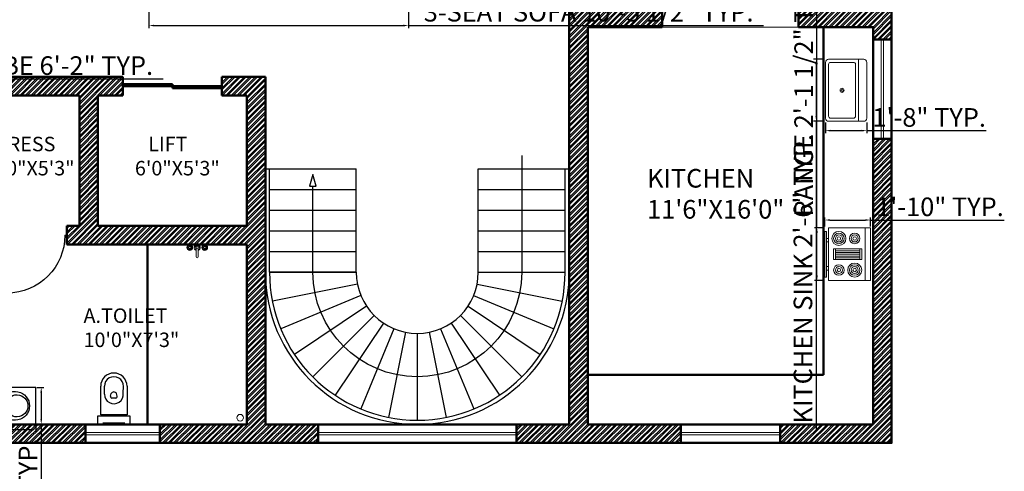
# Model space of a CAD drawing. Units: inches. Extents: x 3590 to 5167, y 65 to 1917.
# Tile 19 of 100: x 3884 to 4360, y 1312 to 1531. Entities that reach past the tile are written whole.
import ezdxf

# ---------------------------------------------------------------- set-up
doc = ezdxf.new("R2010")
doc.units = ezdxf.units.IN
doc.linetypes.add('DASHED', pattern=[0.75, 0.5, -0.25])
for name, color, linetype, lineweight in [('A-ANNO-DIMS', 2, 'Continuous', 18), ('A-AREA-IDEN', 7, 'Continuous', 18), ('A-DOOR', 3, 'Continuous', 25), ('A-FLOR-FIXT', 8, 'Continuous', 18), ('A-FLOR-STRS', 7, 'Continuous', 25), ('A-GLAZ', 4, 'Continuous', 18), ('A-WALL', 7, 'Continuous', 50), ('A-WALL-PATT', 251, 'Continuous', 13), ('S-BEAM-OVHD', 7, 'DASHED', 18)]:
    doc.layers.add(name, color=color, linetype=linetype, lineweight=lineweight)
doc.layers.add('SANTEH', color=7, linetype='Continuous')
doc.styles.get("Standard").update_dxf_attribs({"font": 'arial.ttf'})
doc.dimstyles.new('ISO-25', dxfattribs={"dimtxt": 9, "dimasz": 2.5, "dimexe": 1.25, "dimexo": 0.625, "dimtad": 1, "dimdec": 1, "dimlunit": 3, "dimtxsty": 'Standard', "dimcen": 2.5, "dimadec": 0, "dimazin": 0, "dimtfac": 1, "dimtdec": 1, "dimtmove": 0, "dimatfit": 3, "dimfxl": 1, "dimarcsym": 0})

# ---------------------------------------------------------------- blocks, each defined once
blk = doc.blocks.new('*U1')
blk.add_line((-21, 0), (21, 0))
blk = doc.blocks.new('*U2')
at = {"layer": 'A-FLOR-STRS', "color": 0, "linetype": 'ByBlock', "lineweight": -2, "transparency": 16777216}
for p, rotation in [((4066.16, 1458.03), 101.2499999999998), ((4076.01, 1459), 89.99999999999982), ((4085.86, 1458.03), 78.7499999999998), ((4056.69, 1455.15), 112.4999999999998), ((4095.34, 1455.15), 67.4999999999998), ((4047.96, 1450.49), 123.7499999999997), ((4104.07, 1450.49), 56.24999999999984), ((4040.3, 1444.21), 134.9999999999996), ((4111.72, 1444.21), 44.99999999999992), ((4034.02, 1436.56), 146.2499999999996), ((4118, 1436.56), 33.74999999999991), ((4029.36, 1427.82), 157.4999999999995), ((4122.67, 1427.82), 22.49999999999996), ((4026.48, 1418.35), 168.7499999999995), ((4125.54, 1418.35), 11.25), ((4025.51, 1408.5), 180)]:
    blk.add_blockref('*U1', p, dxfattribs=dict(at, rotation=rotation))
blk.add_blockref('*U1', (4126.51, 1408.5), dxfattribs=at)
blk = doc.blocks.new('Range-Oven - 30 in top')
for p, q in [((0, -3), (30, -3)), ((12, -6), (18, -6)), ((13, -20), (13, -6)), ((14, -6), (14, -20)), ((15, -20), (15, -6)), ((16, -6), (16, -20)), ((17, -20), (17, -6)), ((18, -20), (12, -20)), ((6, -24), (6, -25)), ((8, -25), (8, -24)), ((22, -25), (22, -24)), ((24, -24), (24, -25))]:
    blk.add_line(p, q)
for points in [[(0, -24), (0, 0), (30, 0), (30, -24)], [(12, -21), (12, -5), (18, -5), (18, -21)], [(2, -26), (2, -25), (28, -25), (28, -26)]]:
    blk.add_lwpolyline(points, close=True)
for centre, radius in [((6, -9), 4), ((6, -9), 3), ((6, -9), 2), ((6, -9), 1), ((24, -9), 3), ((24, -9), 2), ((24, -9), 1), ((6, -18), 3), ((6, -18), 2), ((24, -18), 4), ((24, -18), 3), ((24, -18), 2), ((6, -18), 1), ((24, -18), 1)]:
    blk.add_circle(centre, radius)
blk = doc.blocks.new('Sink-single - 30 in top')
blk.add_line((-15, -3.999996), (15, -3.999996))
for points in [[(-13.5, 0), (13.5, 0)], [(-15, -18.499996), (-15, -1.5)], [(15, -1.5), (15, -18.499996)], [(-13.5, -17.499996), (-13.5, -6.499996)], [(-12.5, -5.499996), (12.5, -5.499996)], [(13.5, -6.499996), (13.5, -17.499996)], [(12.5, -18.499996), (-12.5, -18.499996)], [(13.5, -19.999996), (-13.5, -19.999996)]]:
    blk.add_lwpolyline(points)
for radius in [1, 0.5]:
    blk.add_circle((0, -11.999996), radius)
for centre, radius, start, end in [((-13.5, -1.5), 1.5, 90, 180), ((13.5, -1.5), 1.5, 0, 90), ((-12.5, -6.499996), 1, 90, 180), ((12.5, -6.499996), 1, 0, 90), ((-13.5, -18.499996), 1.5, 180, 270), ((-12.5, -17.499996), 1, 180, 270), ((12.5, -17.499996), 1, 270, 0), ((13.5, -18.499996), 1.5, 270, 0)]:
    blk.add_arc(centre, radius, start, end)
blk = doc.blocks.new('D2')
for p, q in [((1, 0), (1, 28)), ((2, 0), (2, 27.98)), ((0, 0), (2, 0)), ((29, 0), (30, 0))]:
    blk.add_line(p, q)
at = {"ltscale": 0.5}
blk.add_arc((1, 0), 28, 0, 90, dxfattribs=at)
blk = doc.blocks.new('y3')
at = {"layer": 'SANTEH', "ltscale": 5}
for p, q in [((38, 131), (38, 521)), ((88, 411), (88, 521)), ((172, 385), (181, 421)), ((263, 385), (254, 421)), ((347, 426), (348, 521)), ((398, 521), (398, 131)), ((244, 358), (191, 358)), ((398, 131), (38, 131)), ((67, 21), (367, 21))]:
    blk.add_line(p, q, dxfattribs=at)
blk.add_lwpolyline([(0, 115), (435, 115), (435, 0), (0, 0), (0, 115)], dxfattribs=at)
for centre, radius, start, end in [((218, 521), 180, 0, 180), ((218, 521), 130, 359.1579, 180), ((218, 411), 130, 180, 5.9855), ((218, 400), 42.2, 30.5234, 149.4766), ((191, 378), 20, 160.5038, 270), ((244, 378), 20, 270, 19.4962)]:
    blk.add_arc(centre, radius, start, end, dxfattribs=at)
blk = doc.blocks.new('r11')
at = {"layer": 'SANTEH', "ltscale": 5}
for p, q in [((0, 0), (600, 0)), ((0, -600), (0, 0)), ((600, 0), (600, -600)), ((210, -50), (390, -50)), ((210, -50), (210, -50)), ((224, -63), (376, -63)), ((224, -113), (224, -63)), ((376, -113), (224, -113)), ((233, -79), (249, -69)), ((233, -98), (233, -79)), ((249, -107), (233, -98)), ((249, -69), (266, -79)), ((266, -98), (249, -107)), ((266, -79), (266, -98)), ((288, -202), (288, -113)), ((312, -113), (312, -202)), ((334, -79), (351, -69)), ((334, -98), (334, -79)), ((351, -107), (334, -98)), ((351, -69), (367, -79)), ((367, -98), (351, -107)), ((367, -79), (367, -98)), ((376, -63), (376, -113)), ((312, -184), (288, -184)), ((312, -202), (288, -202)), ((600, -600), (0, -600))]:
    blk.add_line(p, q, dxfattribs=at)
for centre, radius, start, end in [((300, -266), 234, 112.5, 67.5), ((300, -293), 180, 93.8183, 86.1817)]:
    blk.add_arc(centre, radius, start, end, dxfattribs=at)
blk = doc.blocks.new('Faucet - Bathroom top')
for p, q in [((-4.107, 0.125), (-4.375, 0.125)), ((-3.75, 0.4788), (-3.75, 0.75)), ((-3.5, 0.482), (-3.5, 0.75)), ((-3.1461, 0.125), (-2.875, 0.125)), ((3.143, 0.125), (2.875, 0.125)), ((3.5, 0.4788), (3.5, 0.75)), ((3.75, 0.482), (3.75, 0.75)), ((4.1039, 0.125), (4.375, 0.125)), ((-4.1039, -0.125), (-4.375, -0.125)), ((-3.75, -0.4821), (-3.75, -0.75)), ((-3.5, -0.4789), (-3.5, -0.75)), ((-3.143, -0.125), (-2.875, -0.125)), ((-0.5, -0.8639), (-0.5, -4.5)), ((0.5, -4.5), (0.5, -0.8631)), ((3.1461, -0.125), (2.875, -0.125)), ((3.5, -0.4821), (3.5, -0.75)), ((3.75, -0.4789), (3.75, -0.75)), ((4.107, -0.125), (4.375, -0.125))]:
    blk.add_line(p, q)
for centre, radius in [((-3.625, 0), 1.375), ((-4.625, 0), 0.2795), ((-3.625, 0), 0.5), ((-3.625, 1), 0.2795), ((-2.625, 0), 0.2795), ((0, 0), 0.5), ((3.625, 0), 1.375), ((2.625, 0), 0.2795), ((3.625, 0), 0.5), ((3.625, 1), 0.2795), ((4.625, 0), 0.2795), ((-3.625, -1), 0.2795), ((3.625, -1), 0.2795)]:
    blk.add_circle(centre, radius)
for centre, radius, start, end in [((-3.625, 0), 1, 105.2407, 164.2093), ((-3.625, 0), 1, 16.44125, 74.07887), ((0, 0), 1.5, 289.6514, 250.3603), ((0, 0), 1, 300.3431, 239.7554), ((3.625, 0), 1, 106.12, 164.0884), ((3.625, 0), 1, 16.23422, 73.90469), ((-3.625, 0), 1, 196.2342, 253.9047), ((-3.625, 0), 1, 286.12, 344.0884), ((0, -4.5), 0.5, 180, 0), ((3.625, 0), 1, 196.4413, 254.0789), ((3.625, 0), 1, 285.2407, 344.2093)]:
    blk.add_arc(centre, radius, start, end)
blk = doc.blocks.new('*D290')
at = {"layer": 'A-ANNO-DIMS', "color": 0, "lineweight": -2, "transparency": 16777216}
for p, q in [((3742.44, 1491.53), (3742.44, 1503.26)), ((3744.94, 1502.01), (3813.99, 1502.01)), ((3816.49, 1491.53), (3816.49, 1503.26)), ((3816.49, 1502.01), (3953, 1502.01))]:
    blk.add_line(p, q, dxfattribs=at)
at = {"layer": 'A-ANNO-DIMS', "color": 0, "transparency": 16777216}
for points in [[(3744.94, 1502.43), (3744.94, 1501.59), (3742.44, 1502.01)], [(3813.99, 1502.43), (3813.99, 1501.59), (3816.49, 1502.01)]]:
    blk.add_solid(points, dxfattribs=at)
at = {"layer": 'Defpoints', "color": 0, "transparency": 16777216}
for p in [(3816.49, 1502.01), (3742.44, 1490.9), (3816.49, 1490.9)]:
    blk.add_point(p, dxfattribs=at)
at = {"layer": 'A-ANNO-DIMS', "color": 0, "transparency": 16777216, "insert": (3885.99, 1507.29), "char_height": 9, "attachment_point": 5}
blk.add_mtext('WARDROBE 6\'-2" TYP.', dxfattribs=at)
blk = doc.blocks.new('*D294')
at = {"layer": 'A-ANNO-DIMS', "color": 0, "lineweight": -2, "transparency": 16777216}
for p, q in [((3946.19, 1546.03), (3946.19, 1526.56)), ((4071.76, 1546.03), (4071.76, 1526.56)), ((3948.69, 1527.81), (4069.26, 1527.81)), ((4071.76, 1527.81), (4243.57, 1527.81))]:
    blk.add_line(p, q, dxfattribs=at)
at = {"layer": 'A-ANNO-DIMS', "color": 0, "transparency": 16777216}
for points in [[(3948.69, 1528.23), (3948.69, 1527.4), (3946.19, 1527.81)], [(4069.26, 1528.23), (4069.26, 1527.4), (4071.76, 1527.81)]]:
    blk.add_solid(points, dxfattribs=at)
at = {"layer": 'Defpoints', "color": 0, "transparency": 16777216}
for p in [(3946.19, 1546.65), (4071.76, 1546.65), (4071.76, 1527.81)]:
    blk.add_point(p, dxfattribs=at)
at = {"layer": 'A-ANNO-DIMS', "color": 0, "transparency": 16777216, "insert": (4158.91, 1533.1), "char_height": 9, "attachment_point": 5}
blk.add_mtext('3-SEAT SOFA 10\'-5 1/2" TYP.', dxfattribs=at)
blk = doc.blocks.new('*D306')
at = {"layer": 'A-ANNO-DIMS', "color": 0, "lineweight": -2, "transparency": 16777216}
for p, q in [((3892, 1352.87), (3895.31, 1352.87)), ((3894.06, 1350.37), (3894.06, 1337.5)), ((3892, 1335), (3895.31, 1335)), ((3894.06, 1335), (3894.06, 1193.58))]:
    blk.add_line(p, q, dxfattribs=at)
at = {"layer": 'A-ANNO-DIMS', "color": 0, "transparency": 16777216}
for points in [[(3893.64, 1350.37), (3894.48, 1350.37), (3894.06, 1352.87)], [(3893.64, 1337.5), (3894.48, 1337.5), (3894.06, 1335)]]:
    blk.add_solid(points, dxfattribs=at)
at = {"layer": 'Defpoints', "color": 0, "transparency": 16777216}
for p in [(3891.38, 1352.87), (3891.38, 1335), (3894.06, 1335)]:
    blk.add_point(p, dxfattribs=at)
at = {"layer": 'A-ANNO-DIMS', "color": 0, "transparency": 16777216, "insert": (3888.78, 1263.04), "char_height": 9, "attachment_point": 5, "rotation": 90}
blk.add_mtext('WASH BASIN 1\'-6" TYP.', dxfattribs=at)
blk = doc.blocks.new('*D307')
at = {"layer": 'A-ANNO-DIMS', "color": 0, "lineweight": -2, "transparency": 16777216}
for p, q in [((3873.51, 1334.37), (3873.51, 1331.07)), ((3891.38, 1334.37), (3891.38, 1331.07)), ((3873.51, 1332.32), (3815.75, 1332.32)), ((3888.88, 1332.32), (3876.01, 1332.32))]:
    blk.add_line(p, q, dxfattribs=at)
at = {"layer": 'A-ANNO-DIMS', "color": 0, "transparency": 16777216}
for points in [[(3876.01, 1332.74), (3876.01, 1331.9), (3873.51, 1332.32)], [(3888.88, 1332.74), (3888.88, 1331.9), (3891.38, 1332.32)]]:
    blk.add_solid(points, dxfattribs=at)
at = {"layer": 'Defpoints', "color": 0, "transparency": 16777216}
for p in [(3873.51, 1335), (3891.38, 1335), (3873.51, 1332.32)]:
    blk.add_point(p, dxfattribs=at)
at = {"layer": 'A-ANNO-DIMS', "color": 0, "transparency": 16777216, "insert": (3843.38, 1337.54), "char_height": 9, "attachment_point": 5}
blk.add_mtext('1\'-6" TYP.', dxfattribs=at)
blk = doc.blocks.new('*D308')
at = {"layer": 'A-ANNO-DIMS', "color": 0, "lineweight": -2, "transparency": 16777216}
for p, q in [((4269.39, 1429.97), (4269.39, 1557.29)), ((4272.58, 1429.97), (4268.14, 1429.97)), ((4269.39, 1407.01), (4269.39, 1427.47)), ((4272.58, 1404.51), (4268.14, 1404.51))]:
    blk.add_line(p, q, dxfattribs=at)
at = {"layer": 'A-ANNO-DIMS', "color": 0, "transparency": 16777216}
for points in [[(4268.97, 1427.47), (4269.8, 1427.47), (4269.39, 1429.97)], [(4268.97, 1407.01), (4269.8, 1407.01), (4269.39, 1404.51)]]:
    blk.add_solid(points, dxfattribs=at)
at = {"layer": 'Defpoints', "color": 0, "transparency": 16777216}
for p in [(4269.39, 1429.97), (4273.2, 1429.97), (4273.2, 1404.51)]:
    blk.add_point(p, dxfattribs=at)
at = {"layer": 'A-ANNO-DIMS', "color": 0, "transparency": 16777216, "insert": (4264.11, 1494.88), "char_height": 9, "attachment_point": 5, "rotation": 90}
blk.add_mtext('RANGE 2\'-1 1/2" TYP.', dxfattribs=at)
blk = doc.blocks.new('*D309')
at = {"layer": 'A-ANNO-DIMS', "color": 0, "lineweight": -2, "transparency": 16777216}
for p, q in [((4273.2, 1430.59), (4273.2, 1435.04)), ((4295.27, 1430.59), (4295.27, 1435.04)), ((4275.7, 1433.79), (4292.77, 1433.79)), ((4295.27, 1433.79), (4360.02, 1433.79))]:
    blk.add_line(p, q, dxfattribs=at)
at = {"layer": 'A-ANNO-DIMS', "color": 0, "transparency": 16777216}
for points in [[(4275.7, 1434.2), (4275.7, 1433.37), (4273.2, 1433.79)], [(4292.77, 1434.2), (4292.77, 1433.37), (4295.27, 1433.79)]]:
    blk.add_solid(points, dxfattribs=at)
at = {"layer": 'Defpoints', "color": 0, "transparency": 16777216}
for p in [(4273.2, 1429.97), (4295.27, 1433.79), (4295.27, 1429.97)]:
    blk.add_point(p, dxfattribs=at)
at = {"layer": 'A-ANNO-DIMS', "color": 0, "transparency": 16777216, "insert": (4328.89, 1439.01), "char_height": 9, "attachment_point": 5}
blk.add_mtext('1\'-10" TYP.', dxfattribs=at)
blk = doc.blocks.new('*D310')
at = {"layer": 'A-ANNO-DIMS', "color": 0, "lineweight": -2, "transparency": 16777216}
for p, q in [((4272.91, 1511.51), (4267.78, 1511.51)), ((4269.03, 1509.01), (4269.03, 1484.01)), ((4272.91, 1481.51), (4267.78, 1481.51)), ((4269.03, 1481.51), (4269.03, 1331.79))]:
    blk.add_line(p, q, dxfattribs=at)
at = {"layer": 'A-ANNO-DIMS', "color": 0, "transparency": 16777216}
for points in [[(4268.62, 1509.01), (4269.45, 1509.01), (4269.03, 1511.51)], [(4268.62, 1484.01), (4269.45, 1484.01), (4269.03, 1481.51)]]:
    blk.add_solid(points, dxfattribs=at)
at = {"layer": 'Defpoints', "color": 0, "transparency": 16777216}
for p in [(4273.53, 1511.51), (4269.03, 1481.51), (4273.53, 1481.51)]:
    blk.add_point(p, dxfattribs=at)
at = {"layer": 'A-ANNO-DIMS', "color": 0, "transparency": 16777216, "insert": (4263.76, 1405.4), "char_height": 9, "attachment_point": 5, "rotation": 90}
blk.add_mtext('KITCHEN SINK 2\'-6" TYP.', dxfattribs=at)
blk = doc.blocks.new('*D311')
at = {"layer": 'A-ANNO-DIMS', "color": 0, "lineweight": -2, "transparency": 16777216}
for p, q in [((4273.53, 1480.89), (4273.53, 1475.76)), ((4276.03, 1477.01), (4291.03, 1477.01)), ((4293.53, 1480.89), (4293.53, 1475.76)), ((4293.53, 1477.01), (4351.3, 1477.01))]:
    blk.add_line(p, q, dxfattribs=at)
at = {"layer": 'A-ANNO-DIMS', "color": 0, "transparency": 16777216}
for points in [[(4276.03, 1477.43), (4276.03, 1476.6), (4273.53, 1477.01)], [(4291.03, 1477.43), (4291.03, 1476.6), (4293.53, 1477.01)]]:
    blk.add_solid(points, dxfattribs=at)
at = {"layer": 'Defpoints', "color": 0, "transparency": 16777216}
for p in [(4273.53, 1481.51), (4293.53, 1481.51), (4293.53, 1477.01)]:
    blk.add_point(p, dxfattribs=at)
at = {"layer": 'A-ANNO-DIMS', "color": 0, "transparency": 16777216, "insert": (4323.67, 1482.23), "char_height": 9, "attachment_point": 5}
blk.add_mtext('1\'-8" TYP.', dxfattribs=at)

msp = doc.modelspace()

# ---------------------------------------------------------------- hatches: boundary and pattern name
at = {"layer": 'A-WALL-PATT', "transparency": 33554687}
h = msp.add_hatch(dxfattribs=at)
h.set_pattern_fill('ANSI32', color=256, scale=0.2)
h.paths.add_polyline_path([(3768.51, 1806), (3645.51, 1806), (3645.51, 1785), (3654.51, 1785), (3654.51, 1797), (3671.16, 1797), (3768.51, 1797)])
h.paths.add_polyline_path([(3909.51, 1806), (3816.51, 1806), (3816.51, 1797), (3864.51, 1797), (3864.51, 1791), (3873.51, 1791), (3873.51, 1797), (3909.51, 1797)])
h.paths.add_polyline_path([(4053.51, 1806), (3969.51, 1806), (3969.51, 1797), (4053.51, 1797)])
h.paths.add_polyline_path([(4215.51, 1806), (4113.51, 1806), (4113.51, 1797), (4206.51, 1797), (4206.51, 1791), (4215.51, 1791)])
h.paths.add_polyline_path([(3654.51, 1737), (3645.51, 1737), (3645.51, 1620), (3654.51, 1620), (3654.51, 1650), (3741.51, 1650), (3741.51, 1656), (3654.51, 1656)], flags=17)
h.paths.add_polyline_path([(3873.51, 1755), (3864.51, 1755), (3864.51, 1656), (3771.51, 1656), (3771.51, 1650), (3774.51, 1650), (3774.51, 1554), (3654.51, 1554), (3654.51, 1584), (3645.51, 1584), (3645.51, 1539), (3654.51, 1539), (3654.51, 1545), (3864.51, 1545), (3864.51, 1539), (3873.51, 1539), (3873.51, 1584), (3864.51, 1584), (3864.51, 1554), (3780.51, 1554), (3780.51, 1650), (3864.51, 1650), (3864.51, 1620), (3873.51, 1620)])
h.paths.add_polyline_path([(3654.51, 1491), (3645.51, 1491), (3645.51, 1326), (3810.51, 1326), (3810.51, 1335), (3809.96, 1335), (3654.51, 1335)])
h.paths.add_polyline_path([(3915.51, 1335), (3873.51, 1335), (3873.51, 1352.87), (3873.51, 1422), (3876.51, 1422), (3876.51, 1431), (3864.51, 1431), (3864.51, 1335), (3858.51, 1335), (3858.51, 1326), (3915.51, 1326)])
h.paths.add_polyline_path([(4028.01, 1335), (4002.51, 1335), (4002.51, 1503), (3981.51, 1503), (3981.51, 1494), (3993.51, 1494), (3993.51, 1431), (3921.51, 1431), (3921.51, 1494), (3933.51, 1494), (3933.51, 1503), (3864.51, 1503), (3864.51, 1494), (3912.51, 1494), (3912.51, 1431), (3906.51, 1431), (3906.51, 1422), (3993.51, 1422), (3993.51, 1335), (3951.51, 1335), (3951.51, 1326), (4028.01, 1326)])
h.paths.add_polyline_path([(4203.51, 1335), (4158.51, 1335), (4158.51, 1527), (4194.51, 1527), (4194.51, 1536), (4149.51, 1536), (4149.51, 1335), (4124.01, 1335), (4124.01, 1326), (4203.51, 1326)])
h.paths.add_polyline_path([(4305.51, 1566), (4296.51, 1566), (4296.51, 1536), (4278.64, 1536), (4260.51, 1536), (4260.51, 1527), (4296.51, 1527), (4296.51, 1521), (4305.51, 1521)])
h.paths.add_polyline_path([(4305.51, 1473), (4296.51, 1473), (4296.51, 1335), (4251.51, 1335), (4251.51, 1326), (4305.51, 1326)])
h.paths.add_polyline_path([(4305.51, 1677), (4215.51, 1677), (4215.51, 1743), (4206.51, 1743), (4206.51, 1677), (4149.51, 1677), (4149.51, 1668), (4296.51, 1668), (4296.51, 1638), (4305.51, 1638)])

# ---------------------------------------------------------------- linework, layer by layer
at = {"layer": 'A-FLOR-FIXT'}
msp.add_circle((3990.31, 1338.21), 1.6, dxfattribs=at)
at = {"layer": 'A-FLOR-STRS'}
for p, q in [((4002.51, 1458.5), (4046.51, 1458.5)), ((4004.51, 1408.5), (4004.51, 1458.5)), ((4046.51, 1408.5), (4046.51, 1458.5)), ((4105.51, 1408.5), (4105.51, 1458.5)), ((4105.51, 1458.5), (4149.51, 1458.5)), ((4147.51, 1408.5), (4147.51, 1458.5)), ((4004.51, 1448.5), (4046.51, 1448.5)), ((4105.51, 1448.5), (4147.51, 1448.5)), ((4004.51, 1438.5), (4046.51, 1438.5)), ((4105.51, 1438.5), (4147.51, 1438.5)), ((4004.51, 1428.5), (4046.51, 1428.5)), ((4105.51, 1428.5), (4147.51, 1428.5)), ((4004.51, 1418.5), (4046.51, 1418.5)), ((4105.51, 1418.5), (4147.51, 1418.5)), ((4004.51, 1408.5), (4046.51, 1408.5))]:
    msp.add_line(p, q, dxfattribs=at)
msp.add_lwpolyline([(4126.51, 1464.94), (4126.51, 1408.5, -1), (4025.51, 1408.5), (4025.51, 1450.11)], format="xyb", dxfattribs=at)
msp.add_lwpolyline([(4025.51, 1455.87), (4023.88, 1450.11), (4027.15, 1450.11)], close=True, dxfattribs=at)
for radius in [73.5, 71.5, 29.5]:
    msp.add_arc((4076.01, 1408.5), radius, 180, 0, dxfattribs=at)
at = {"layer": 'A-GLAZ'}
for p, q in [((4300.51, 1473), (4300.51, 1521)), ((4301.51, 1473), (4301.51, 1521)), ((3951.51, 1331), (3915.51, 1331)), ((3951.51, 1330), (3915.51, 1330)), ((4124.01, 1331), (4028.01, 1331)), ((4124.01, 1330), (4028.01, 1330)), ((4251.51, 1331), (4203.51, 1331)), ((4251.51, 1330), (4203.51, 1330))]:
    msp.add_line(p, q, dxfattribs=at)
at = {"layer": 'A-WALL'}
for p, q in [((4149.51, 1335), (4149.51, 1536)), ((4194.51, 1527), (4194.51, 1536)), ((4260.51, 1527), (4260.51, 1536)), ((4158.51, 1335), (4158.51, 1527)), ((4194.51, 1527), (4158.51, 1527)), ((4296.51, 1527), (4260.51, 1527)), ((4272.51, 1527), (4272.51, 1359)), ((4296.51, 1527), (4296.51, 1335)), ((4305.51, 1521), (4296.51, 1521)), ((3933.51, 1503), (3864.51, 1503)), ((3933.51, 1494), (3933.51, 1503)), ((4002.51, 1503), (3981.51, 1503)), ((3981.51, 1494), (3981.51, 1503)), ((4002.51, 1335), (4002.51, 1503)), ((3933.51, 1499.5), (3957.51, 1499.5)), ((3933.51, 1498.5), (3981.51, 1498.5)), ((3957.51, 1499.5), (3957.51, 1497.5)), ((3957.51, 1497.5), (3981.51, 1497.5)), ((3912.51, 1494), (3864.51, 1494)), ((3912.51, 1431), (3912.51, 1494)), ((3921.51, 1431), (3921.51, 1494)), ((3933.51, 1494), (3921.51, 1494)), ((3993.51, 1494), (3981.51, 1494)), ((3993.51, 1431), (3993.51, 1494)), ((4305.51, 1473), (4296.51, 1473)), ((3912.51, 1431), (3906.51, 1431)), ((3906.51, 1422), (3906.51, 1431)), ((3993.51, 1431), (3921.51, 1431)), ((3993.51, 1422), (3906.51, 1422)), ((3945.51, 1335), (3945.51, 1422)), ((3993.51, 1335), (3993.51, 1422)), ((4272.51, 1359), (4158.51, 1359)), ((3993.51, 1335), (3873.51, 1335)), ((3915.51, 1335), (3915.51, 1326)), ((3951.51, 1335), (3951.51, 1326)), ((4149.51, 1335), (4002.51, 1335)), ((4028.01, 1335), (4028.01, 1326)), ((4124.01, 1335), (4124.01, 1326)), ((4296.51, 1335), (4158.51, 1335)), ((4203.51, 1335), (4203.51, 1326)), ((4251.51, 1335), (4251.51, 1326))]:
    msp.add_line(p, q, dxfattribs=at)
msp.add_lwpolyline([(4305.51, 1677), (4305.51, 1326), (3645.51, 1326), (3645.51, 1806), (4215.51, 1806)], dxfattribs=at)
at = {"layer": 'S-BEAM-OVHD', "ltscale": 0.5}
msp.add_line((4194.51, 1527), (4260.51, 1527), dxfattribs=at)

# ---------------------------------------------------------------- block references
at = {"layer": 'A-DOOR', "xscale": -1, "rotation": 180}
msp.add_blockref('D2', (3876.51, 1426.5), dxfattribs=at)
at = {"layer": 'A-FLOR-FIXT', "rotation": 270}
msp.add_blockref('Sink-single - 30 in top', (4293.53, 1496.51), dxfattribs=at)
at = {"layer": 'A-FLOR-FIXT'}
for name, p, xscale, yscale, zscale, rotation in [('Range-Oven - 30 in top', (4295.27, 1404.51), -0.8485281468519549, 0.8485281468519549, 0.8485281468519549, 270), ('r11', (3873.51, 1352.87), -0.0297800069284724, 0.0297800069284724, 0.0297800069284724, 90)]:
    msp.add_blockref(name, p, dxfattribs=dict(at, xscale=xscale, yscale=yscale, zscale=zscale, rotation=rotation))
msp.add_blockref('Faucet - Bathroom top', (3969.55, 1420.5), dxfattribs=at)
at = {"layer": 'A-FLOR-FIXT', "xscale": 0.0353848906415677, "yscale": 0.0353848906415677, "zscale": 0.0353848906415677}
msp.add_blockref('y3', (3921.48, 1335), dxfattribs=at)
at = {"layer": 'A-FLOR-STRS', "xscale": -1, "rotation": 180}
msp.add_blockref('*U2', (0, 2817), dxfattribs=at)

# ---------------------------------------------------------------- texts
at = {"layer": 'A-AREA-IDEN', "attachment_point": 1}
for s, insert, char_height in [('{\\fTimes New Roman|b0|i0|c0|p18; DRESS\\P4\'0"X5\'3"}', (3869.13, 1474.03), 7), ('{\\fTimes New Roman|b0|i0|c0|p18;   LIFT\\P6\'0"X5\'3"}', (3939.39, 1474.03), 7), ('{\\fTimes New Roman|b0|i0|c0|p18;KITCHEN\\P11\'6"X16\'0"}', (4187.19, 1458.47), 9), ('{\\fTimes New Roman|b0|i0|c0|p18;A.TOILET\\P10\'0"X7\'3"}', (3914.52, 1391.04), 7)]:
    msp.add_mtext_dynamic_manual_height_columns(s, width=67.3508, gutter_width=12.5, heights=[0], dxfattribs=dict(at, insert=insert, char_height=char_height))

# ---------------------------------------------------------------- dimensions: what is measured, and where the dimension line sits
at = {"layer": 'A-ANNO-DIMS'}
for base, p1, p2, text, picture, middle in [((4071.76, 1527.81), (3946.19, 1546.65), (4071.76, 1546.65), '3-SEAT SOFA <> TYP.', '*D294', (4158.91, 1533.1)), ((3816.4865, 1502.0094), (3742.4429, 1490.9029), (3816.4865, 1490.9029), 'WARDROBE <> TYP.', '*D290', (3885.9942, 1507.291)), ((4293.53, 1477.01), (4273.53, 1481.51), (4293.53, 1481.51), '<> TYP.', '*D311', (4323.67, 1482.23)), ((4295.27, 1433.79), (4273.2, 1429.97), (4295.27, 1429.97), '<> TYP.', '*D309', (4328.89, 1439.01))]:
    dim = msp.add_linear_dim(base=base, p1=p1, p2=p2, text=text, dimstyle='ISO-25', override={"dimdec": 1, "dimlfac": 1, "dimrnd": 0, "dimzin": 1, "dimdsep": 46, "dimlunit": 4, "dimfrac": 2}, dxfattribs=at)
    dim.commit()
    dim.dimension.update_dxf_attribs({"geometry": picture, "text_midpoint": middle})
for base, p1, p2, angle, text, picture, middle in [((4269.39, 1429.97), (4273.2, 1404.51), (4273.2, 1429.97), 90, 'RANGE <> TYP.', '*D308', (4264.11, 1494.88)), ((4269.03, 1481.51), (4273.53, 1511.51), (4273.53, 1481.51), 270, 'KITCHEN SINK <> TYP.', '*D310', (4263.76, 1405.4)), ((3873.51, 1332.32), (3891.38, 1335), (3873.51, 1335), 180, '<> TYP.', '*D307', (3843.38, 1337.54)), ((3894.06, 1335), (3891.38, 1352.87), (3891.38, 1335), 270, 'WASH BASIN <> TYP.', '*D306', (3888.78, 1263.04))]:
    dim = msp.add_linear_dim(base=base, p1=p1, p2=p2, angle=angle, text=text, dimstyle='ISO-25', override={"dimdec": 1, "dimlfac": 1, "dimrnd": 0, "dimzin": 1, "dimdsep": 46, "dimlunit": 4, "dimfrac": 2}, dxfattribs=at)
    dim.commit()
    dim.dimension.update_dxf_attribs({"geometry": picture, "text_midpoint": middle})

doc.saveas('drawing.dxf')
